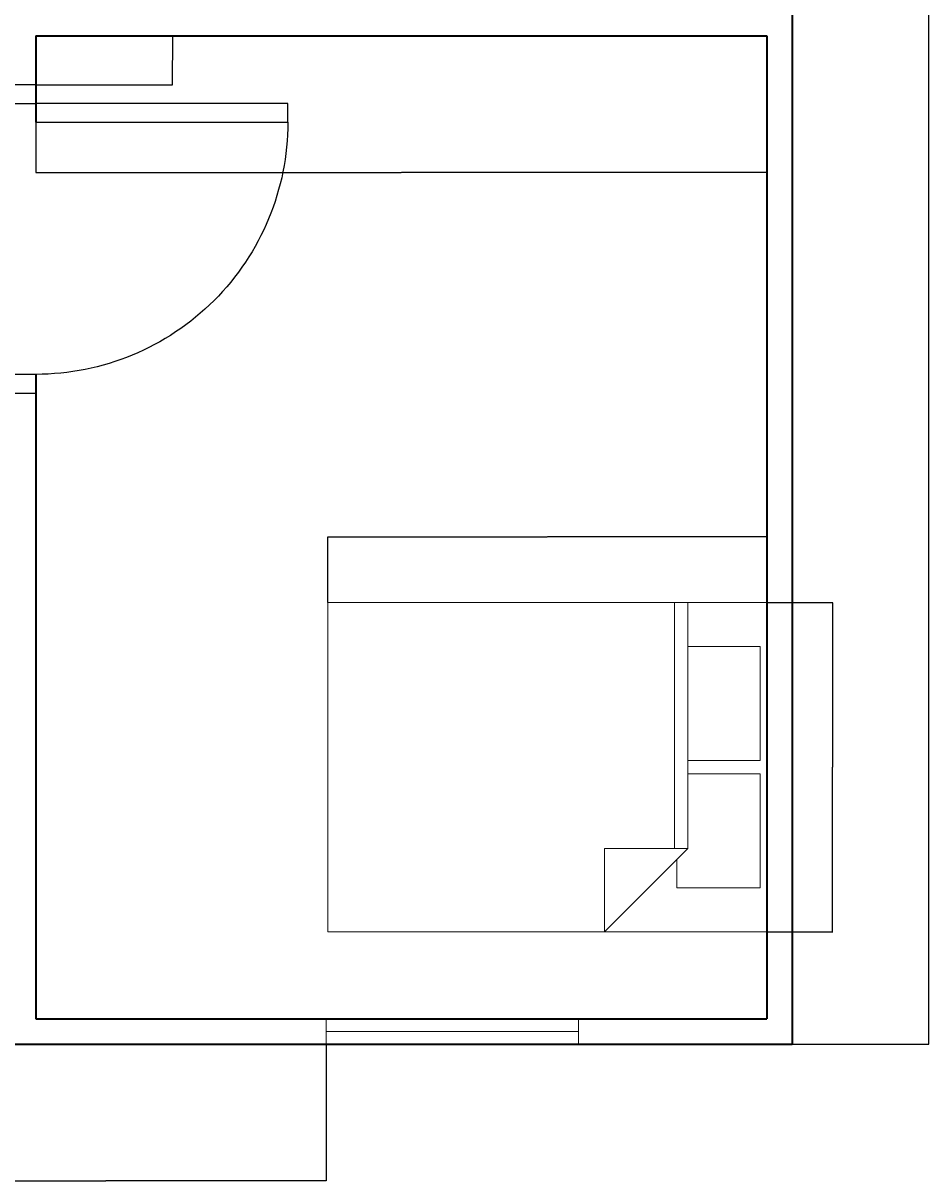
# Model space of a CAD drawing. Units: millimetres. Extents: x 1426 to 11512, y -8522 to 2664.
# Tile 1 of 4: x 7919 to 11512, y -8522 to -3929. Entities that reach past the tile are written whole.
import ezdxf

# ---------------------------------------------------------------- set-up
doc = ezdxf.new("R2010")
doc.units = ezdxf.units.MM
for name, color, linetype, lineweight in [('A-ANNO-DIMS', 2, 'Continuous', 18), ('A-DOOR', 3, 'Continuous', 25), ('A-FURN', 8, 'Continuous', 18), ('A-GLAZ', 4, 'Continuous', 18), ('A-WALL', 7, 'Continuous', 35)]:
    doc.layers.add(name, color=color, linetype=linetype, lineweight=lineweight)
doc.styles.get("Standard").update_dxf_attribs({"font": 'arial.ttf'})
doc.dimstyles.get("Standard").update_dxf_attribs({"dimtxt": 0.18, "dimasz": 0.18, "dimexe": 0.18, "dimexo": 0.0625, "dimgap": 0.09, "dimtad": 0, "dimtih": 1, "dimtoh": 1, "dimdec": 4, "dimzin": 0, "dimdsep": 46, "dimtxsty": 'Standard', "dimcen": 0.09, "dimadec": 0, "dimazin": 0, "dimtfac": 1, "dimtdec": 4, "dimtofl": 0, "dimtmove": 0, "dimatfit": 3, "dimfxl": 1, "dimtolj": 1, "dimtzin": 0, "dimarcsym": 0})

# ---------------------------------------------------------------- blocks, each defined once
blk = doc.blocks.new('Bed - Queen')
for p, q in [((0, -80.00003000000002), (0, 0)), ((0, 0), (59.99998999999999, 0)), ((59.99998999999999, 0), (59.99998999999999, -80.00003000000002)), ((7.99999, -1.200000000000017), (28.79998, -1.200000000000017)), ((7.99999, -14.4), (7.99999, -1.200000000000017)), ((28.79998, -1.200000000000017), (28.79998, -14.4)), ((31.19999, -1.200000000000017), (51.99999000000001, -1.200000000000017)), ((31.19999, -14.4), (31.19999, -1.200000000000017)), ((51.99999000000001, -1.200000000000017), (51.99999000000001, -16.4)), ((0, -14.4), (44.79999999999999, -14.4)), ((59.99998999999999, -29.60000000000001), (44.79999999999999, -14.4)), ((44.79999999999999, -14.4), (44.79999999999999, -29.60000000000001)), ((44.79999999999999, -16.80000000000001), (0, -16.80000000000001)), ((51.99999000000001, -16.4), (46.79936, -16.4)), ((44.79999999999999, -29.60000000000001), (59.99998999999999, -29.60000000000001)), ((59.99998999999999, -80.00003000000002), (0, -80.00003000000002))]:
    blk.add_line(p, q)
blk = doc.blocks.new('DOOR-SINGLE-1000')
for p, q in [((-0.0002449408875691, 999.9999577541435), (-0.0002449408875691, 1099.999957754143)), ((-0.0002449408875691, 1099.999957754143), (74.19975505911316, 1099.999957754143)), ((74.19975505911316, 1099.999957754143), (74.19975505911316, 999.9999577541435)), ((1148.399755059116, 999.999957754143), (1148.399755059116, 1099.999957754143)), ((1148.399755059116, 1099.999957754143), (1222.599755059116, 1099.999957754143)), ((1222.599755059116, 1099.999957754143), (1222.599755059116, 999.9999577541435)), ((74.19975505911316, 999.9999577541435), (-0.0002449408875691, 999.9999577541435)), ((74.19975505911316, 999.9999577541435), (148.3997550591139, 999.9999577541435)), ((74.19975505911316, -4.22458564344e-05), (74.19975505911316, 999.9999577541435)), ((148.3997550591139, 999.9999577541435), (148.3997550591139, -4.22458564344e-05)), ((1222.599755059116, 999.999957754143), (1148.399755059116, 999.999957754143)), ((148.3997550591139, -4.22458564344e-05), (74.19975505911316, -4.22458564344e-05))]:
    blk.add_line(p, q)
blk.add_arc((148.3997550591157, 999.9999577541435), 999.9999999999998, 270, 0)
blk = doc.blocks.new('WIN-1000')
for p, q in [((-0.0003881192678818, 99.99995775414573), (999.999611880732, 99.99995775414573)), ((-0.0003881192678818, -4.22458542744e-05), (-0.0003881192678818, 99.99995775414573)), ((999.999611880732, 99.99995775414573), (999.999611880732, -4.22458542744e-05)), ((-0.0003881192678818, 49.99995775414572), (999.999611880732, 49.99995775414572)), ((999.999611880732, -4.22458542744e-05), (-0.0003881192678818, -4.22458542744e-05))]:
    blk.add_line(p, q)
blk = doc.blocks.new('*D24')
at = {"layer": 'A-ANNO-DIMS', "color": 0, "lineweight": -2, "transparency": 16777216}
for p, q in [((9127.747412128118, -6227.857895482565), (9127.747412128118, -5966.571709643759)), ((9127.927412128118, -5966.75170964376), (9997.678838775886, -5966.75170964376)), ((10868.69198438682, -5966.75170964376), (9998.94055773905, -5966.75170964376)), ((10868.87198438682, -6227.857895482565), (10868.87198438682, -5966.571709643759))]:
    blk.add_line(p, q, dxfattribs=at)
at = {"layer": 'A-ANNO-DIMS', "color": 0, "transparency": 16777216}
for points in [[(9127.927412128118, -5966.72170964376), (9127.927412128118, -5966.781709643759), (9127.747412128118, -5966.75170964376)], [(10868.69198438682, -5966.72170964376), (10868.69198438682, -5966.781709643759), (10868.87198438682, -5966.75170964376)]]:
    blk.add_solid(points, dxfattribs=at)
at = {"layer": 'Defpoints', "color": 0, "transparency": 16777216}
for p in [(10868.87198438682, -5966.75170964376), (9127.747412128118, -6227.920395482565), (10868.87198438682, -6227.920395482565)]:
    blk.add_point(p, dxfattribs=at)
at = {"layer": 'A-ANNO-DIMS', "color": 0, "transparency": 16777216, "insert": (9998.309698257468, -5966.75170964376), "char_height": 0.18, "attachment_point": 5}
blk.add_mtext('\\A1;BED 1741', dxfattribs=at)
blk = doc.blocks.new('*D25')
at = {"layer": 'A-ANNO-DIMS', "color": 0, "lineweight": -2, "transparency": 16777216}
for p, q in [((10868.93448438682, -6227.920395482569), (11130.22067022563, -6227.920395482569)), ((11130.04067022563, -6228.100395482569), (11130.04067022563, -6880.659791884454)), ((11130.04067022563, -7533.583117345003), (11130.04067022563, -6881.023720943118)), ((10868.93448438682, -7533.763117345003), (11130.22067022563, -7533.763117345003))]:
    blk.add_line(p, q, dxfattribs=at)
at = {"layer": 'A-ANNO-DIMS', "color": 0, "transparency": 16777216}
for points in [[(11130.01067022563, -6228.100395482569), (11130.07067022563, -6228.100395482569), (11130.04067022563, -6227.920395482569)], [(11130.01067022563, -7533.583117345003), (11130.07067022563, -7533.583117345003), (11130.04067022563, -7533.763117345003)]]:
    blk.add_solid(points, dxfattribs=at)
at = {"layer": 'Defpoints', "color": 0, "transparency": 16777216}
for p in [(10868.87198438682, -6227.920395482569), (10868.87198438682, -7533.763117345003), (11130.04067022563, -7533.763117345003)]:
    blk.add_point(p, dxfattribs=at)
at = {"layer": 'A-ANNO-DIMS', "color": 0, "transparency": 16777216, "insert": (11130.04067022563, -6880.841756413788), "char_height": 0.18, "attachment_point": 5}
blk.add_mtext('\\A1;1306', dxfattribs=at)
blk = doc.blocks.new('*D38')
at = {"layer": 'A-ANNO-DIMS', "color": 0, "lineweight": -2, "transparency": 16777216}
for p, q in [((10968.934484, 2120.944958000001), (11511.55198400001, 2120.944958000002)), ((11511.371984, 2120.764958000002), (11511.371984, -2928.87313886221)), ((11511.37198400001, -7978.875042000002), (11511.371984, -2929.236945137791)), ((10968.934484, -7979.055042000003), (11511.55198400001, -7979.055042000003))]:
    blk.add_line(p, q, dxfattribs=at)
at = {"layer": 'A-ANNO-DIMS', "color": 0, "transparency": 16777216}
for points in [[(11511.341984, 2120.764958000002), (11511.401984, 2120.764958000002), (11511.371984, 2120.944958000002)], [(11511.341984, -7978.875042000002), (11511.40198400001, -7978.875042000002), (11511.37198400001, -7979.055042000003)]]:
    blk.add_solid(points, dxfattribs=at)
at = {"layer": 'Defpoints', "color": 0, "transparency": 16777216}
for p in [(10968.871984, 2120.944958000001), (10968.871984, -7979.055042000003), (11511.37198400001, -7979.055042000003)]:
    blk.add_point(p, dxfattribs=at)
at = {"layer": 'A-ANNO-DIMS', "color": 0, "transparency": 16777216, "insert": (11511.371984, -2929.055042000004), "char_height": 0.18, "attachment_point": 5}
blk.add_mtext('\\A1;10100', dxfattribs=at)
blk = doc.blocks.new('*D42')
at = {"layer": 'A-ANNO-DIMS', "color": 0, "lineweight": -2, "transparency": 16777216}
for p, q in [((7968.871984, -3979.117542), (7968.871984, -4521.735042)), ((10868.871984, -3979.117542), (10868.871984, -4521.735042)), ((7969.051984, -4521.555042), (9418.511983999999, -4521.555042)), ((10868.691984, -4521.555042), (9419.231983999998, -4521.555042))]:
    blk.add_line(p, q, dxfattribs=at)
at = {"layer": 'A-ANNO-DIMS', "color": 0, "transparency": 16777216}
for points in [[(7969.051984, -4521.525042), (7969.051984, -4521.585041999999), (7968.871984, -4521.555042)], [(10868.691984, -4521.525042), (10868.691984, -4521.585041999999), (10868.871984, -4521.555042)]]:
    blk.add_solid(points, dxfattribs=at)
at = {"layer": 'Defpoints', "color": 0, "transparency": 16777216}
for p in [(7968.871984, -3979.055042), (10868.871984, -3979.055042), (7968.871984, -4521.555042)]:
    blk.add_point(p, dxfattribs=at)
at = {"layer": 'A-ANNO-DIMS', "color": 0, "transparency": 16777216, "insert": (9418.871984, -4521.555042), "char_height": 0.18, "attachment_point": 5}
blk.add_mtext('\\A1;2900', dxfattribs=at)
blk = doc.blocks.new('*D53')
at = {"layer": 'A-ANNO-DIMS', "color": 0, "lineweight": -2, "transparency": 16777216}
for p, q in [((7372.550530000001, -7979.117542), (7372.550530000001, -8521.735042)), ((9121.359612, -7979.117542), (9121.359612, -8521.735041999998)), ((7372.730530000001, -8521.555042000002), (8246.49972993588, -8521.555042000002)), ((9121.179612, -8521.555041999998), (8247.41041206412, -8521.555042000002))]:
    blk.add_line(p, q, dxfattribs=at)
at = {"layer": 'A-ANNO-DIMS', "color": 0, "transparency": 16777216}
for points in [[(7372.730530000001, -8521.525042000001), (7372.730530000001, -8521.585042000002), (7372.550530000001, -8521.555042000002)], [(9121.179612, -8521.525041999997), (9121.179612, -8521.585041999999), (9121.359612, -8521.555041999998)]]:
    blk.add_solid(points, dxfattribs=at)
at = {"layer": 'Defpoints', "color": 0, "transparency": 16777216}
for p in [(7372.550530000001, -7979.055042), (9121.359612, -7979.055042), (7372.550530000001, -8521.555042000002)]:
    blk.add_point(p, dxfattribs=at)
at = {"layer": 'A-ANNO-DIMS', "color": 0, "transparency": 16777216, "insert": (8246.955071, -8521.555042000002), "char_height": 0.18, "attachment_point": 5}
blk.add_mtext('\\A1;1748.8', dxfattribs=at)
blk = doc.blocks.new('*D71')
at = {"layer": 'A-ANNO-DIMS', "color": 0, "lineweight": -2, "transparency": 16777216}
for p, q in [((7968.934484000005, -3979.055042000002), (8511.551984000007, -3979.055042000002)), ((8511.371984000007, -3979.235042000002), (8511.371984000007, -4076.268540362212)), ((8511.371984000009, -4173.665845000001), (8511.371984000007, -4076.632346637792)), ((7968.934484000005, -4173.845845000001), (8511.551984000009, -4173.845845000001))]:
    blk.add_line(p, q, dxfattribs=at)
at = {"layer": 'A-ANNO-DIMS', "color": 0, "transparency": 16777216}
for points in [[(8511.341984000006, -3979.235042000002), (8511.401984000007, -3979.235042000002), (8511.371984000007, -3979.055042000002)], [(8511.341984000008, -4173.665845000001), (8511.40198400001, -4173.665845000001), (8511.371984000009, -4173.845845000001)]]:
    blk.add_solid(points, dxfattribs=at)
at = {"layer": 'Defpoints', "color": 0, "transparency": 16777216}
for p in [(7968.871984000005, -3979.055042000002), (7968.871984000005, -4173.845845000001), (8511.371984000009, -4173.845845000001)]:
    blk.add_point(p, dxfattribs=at)
at = {"layer": 'A-ANNO-DIMS', "color": 0, "transparency": 16777216, "insert": (8511.371984000005, -4076.450443500003), "char_height": 0.18, "attachment_point": 5}
blk.add_mtext('\\A1;194.8', dxfattribs=at)

msp = doc.modelspace()

# ---------------------------------------------------------------- linework, layer by layer
at = {"layer": 'A-WALL'}
for p, q in [((10968.87198438682, 2120.944957754144), (10968.87198438681, -7979.055042245858)), ((7968.87198438682, -3979.055042245857), (7968.87198438682, -4322.24584538863)), ((7968.871984386819, -3979.055042245857), (10868.87198438682, -3979.055042245857)), ((10868.87198438682, -3979.055042245857), (10868.87198438682, -7879.055042245855)), ((7968.87198438682, -5322.245845388632), (7968.87198438682, -7879.055042245855)), ((7968.87198438682, -7879.055042245855), (10868.87198438681, -7879.055042245855)), ((7298.350529566508, -7979.055042245857), (10968.87198438681, -7979.055042245857))]:
    msp.add_line(p, q, dxfattribs=at)

# ---------------------------------------------------------------- block references
at = {"layer": 'A-DOOR', "extrusion": (0, 0, -1), "zscale": -1, "rotation": 269.9999999999998}
msp.add_blockref('DOOR-SINGLE-1000', (-8968.87194214096, -4173.846090329516), dxfattribs=at)
at = {"layer": 'A-FURN', "xscale": 21.7640489917154, "yscale": 21.7640489917154, "zscale": 21.7640489917154, "rotation": 270}
msp.add_blockref('Bed - Queen', (10868.87198438682, -6227.920395482565), dxfattribs=at)
at = {"layer": 'A-GLAZ'}
msp.add_blockref('WIN-1000', (9121.36, -7979.055000000001), dxfattribs=at)

# ---------------------------------------------------------------- dimensions: what is measured, and where the dimension line sits
at = {"layer": 'A-ANNO-DIMS'}
for base, p1, p2, angle, override, picture, middle in [((11511.37198400001, -7979.055042000003), (10968.871984, 2120.944958), (10968.871984, -7979.055042), 90, {"dimdec": 0, "dimlfac": 1, "dimrnd": 0, "dimzin": 0, "dimdsep": 46, "dimlunit": 2}, '*D38', (11511.371984, -2929.055042000004)), ((7968.871984, -4521.555042), (10868.871984, -3979.055042), (7968.871984, -3979.055042), 180, {"dimdec": 0, "dimlfac": 1, "dimrnd": 0, "dimzin": 0, "dimdsep": 46, "dimlunit": 2}, '*D42', (9418.871984, -4521.555042)), ((8511.371984000009, -4173.845845000001), (7968.871984, -3979.055042), (7968.871984, -4173.845844999999), 269.9999999999993, {"dimdec": 1, "dimlfac": 1, "dimrnd": 0, "dimzin": 0, "dimdsep": 46, "dimlunit": 2}, '*D71', (8511.371984000005, -4076.450443500003)), ((11130.04067022563, -7533.763117345003), (10868.87198438682, -6227.920395482565), (10868.87198438682, -7533.763117344999), 270, {"dimdec": 0, "dimlfac": 1, "dimrnd": 0, "dimzin": 0, "dimdsep": 46, "dimlunit": 2}, '*D25', (11130.04067022563, -6880.841756413788)), ((7372.550530000001, -8521.555042000002), (9121.359612, -7979.055042), (7372.550530000001, -7979.055042), 180.0000000000001, {"dimdec": 1, "dimlfac": 1, "dimrnd": 0, "dimzin": 0, "dimdsep": 46, "dimlunit": 2}, '*D53', (8246.955071, -8521.555042000002))]:
    dim = msp.add_linear_dim(base=base, p1=p1, p2=p2, angle=angle, dimstyle='Standard', override=override, dxfattribs=at)
    dim.commit()
    dim.dimension.update_dxf_attribs({"geometry": picture, "text_midpoint": middle})
dim = msp.add_linear_dim(base=(10868.87198438682, -5966.75170964376), p1=(9127.747412128118, -6227.920395482565), p2=(10868.87198438682, -6227.920395482565), text='BED <>', dimstyle='Standard', override={"dimdec": 0, "dimlfac": 1, "dimrnd": 0, "dimzin": 0, "dimdsep": 46, "dimlunit": 2}, dxfattribs=at)
dim.commit()
dim.dimension.update_dxf_attribs({"geometry": '*D24', "text_midpoint": (9998.309698257468, -5966.75170964376)})

doc.saveas('drawing.dxf')
